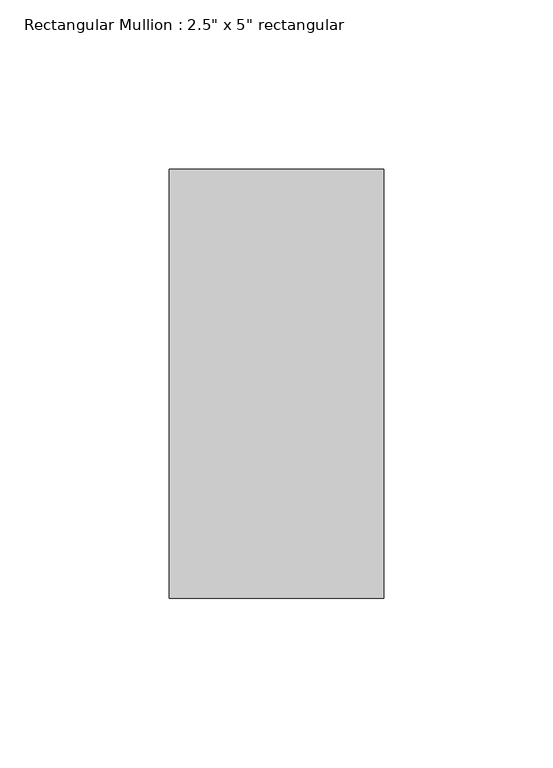
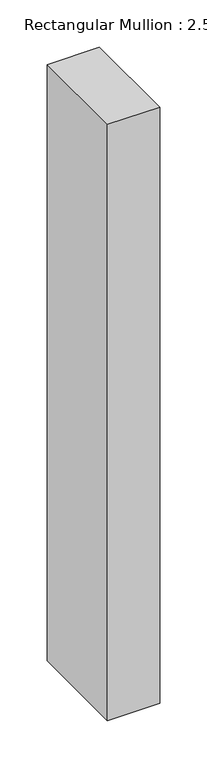
"""IFC4 building model written with IfcOpenShell, lengths in millimetres: member geometry."""

from ifc_helpers import new_model, si_unit, frame, origin, place, context, project, spatial, polyline, outline, extrude, source, transform, mapped, element, save


def member_1407b1c2(model_context):
    return source(origin(), model_context, "Body", "SweptSolid", [
        extrude(outline(polyline([(0.0, 63.5), (0.0, -63.5), (-63.5, -63.5), (-63.5, 63.5), (0.0, 63.5)])), frame((0.0, 0.0, -768.5795173), z_axis=(0.0, 0.0, 1.0), x_axis=(1.0, 0.0, 0.0)), (0.0, 0.0, 1.0), 768.5795173),
    ])


if __name__ == "__main__":
    model = new_model("IFC4")
    model_context = context("Model", 3, world=origin())
    ifc_project = project(units=[si_unit("LENGTHUNIT", "METRE", prefix="MILLI")], contexts=[model_context])
    site = spatial("IfcSite", under=ifc_project)
    building = spatial("IfcBuilding", under=site)
    placement = place(None, origin())
    member_shape = member_1407b1c2(model_context)
    element("IfcMember", 1, ObjectType="Rectangular Mullion : 2.5\" x 5\" rectangular", at=placement, inside=building, context=model_context, shape_type="MappedRepresentation", body=[
        mapped(member_shape, transform((0.0, 0.0, 0.0), x_axis=(1.0, 0.0, 0.0), y_axis=(0.0, 1.0, 0.0), z_axis=(0.0, 0.0, 1.0))),
    ])
    save(model, "model.ifc")

# Revit data of these elements
# Type "Rectangular Mullion : 2.5\" x 5\" rectangular"
#   built-in parameter 1007304 = 0.416667 (stored number, unit not read)
#   built-in parameter 1007301 = 0.104167 (stored number, unit not read)
#   built-in parameter 1007300 = 0.104167 (stored number, unit not read)
# Element 1 (IfcMember, "Rectangular Mullion : 2.5\" x 5\" rectangular")
#   Materials on its faces: "Aluminum"
# Materials
#   "Aluminum": class "Metal", colour RGB 247 247 247, transparency 0, Description = "Aluminum 6061", Cost = 0
